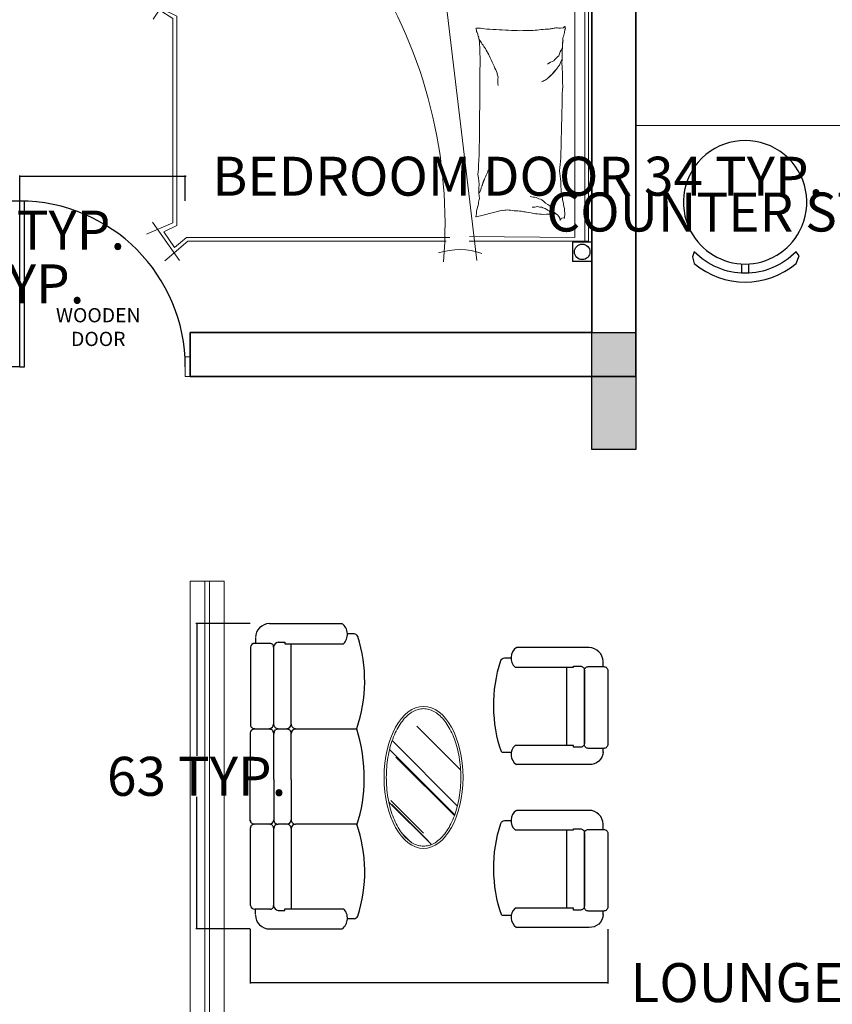
# Model space of a CAD drawing. Units: inches. Extents: x -48 to 50072, y 0 to 21068.
# Tile 68 of 75: x 925 to 1092, y 803 to 1005. Entities that reach past the tile are written whole.
import ezdxf

# ---------------------------------------------------------------- set-up
doc = ezdxf.new("R2010")
doc.units = ezdxf.units.IN
doc.header["$MEASUREMENT"] = 0
for name, color, linetype in [('2D', 7, 'Continuous'), ('BLOCKS', 7, 'Continuous'), ('家具1', 1, 'Continuous'), ('家具１', 1, 'Continuous')]:
    doc.layers.add(name, color=color, linetype=linetype)
for name, color, linetype, lineweight in [('A-ANNO-DIMS', 2, 'Continuous', 18), ('A-COLS', 1, 'Continuous', 35), ('A-DOOR', 4, 'Continuous', 18), ('A-FLOR-CASE', 9, 'Continuous', 18), ('A-FLOR-SCRN', 32, 'Continuous', 18), ('A-WALL', 7, 'Continuous', 35), ('FURNITURE', 44, 'Continuous', 18)]:
    doc.layers.add(name, color=color, linetype=linetype, lineweight=lineweight)
doc.styles.get("Standard").update_dxf_attribs({"font": 'arial.ttf'})
doc.dimstyles.get("Standard").update_dxf_attribs({"dimtxt": 8, "dimasz": 0.18, "dimexe": 0.18, "dimexo": 0.0625, "dimgap": 0.09, "dimtad": 0, "dimtih": 1, "dimtoh": 1, "dimdec": 1, "dimzin": 0, "dimdsep": 46, "dimlunit": 4, "dimtxsty": 'Standard', "dimblk": 'ARCHTICK', "dimcen": 0.09, "dimadec": 0, "dimazin": 0, "dimtfac": 1, "dimtdec": 1, "dimtofl": 0, "dimtmove": 0, "dimatfit": 3, "dimldrblk": 'ARCHTICK', "dimfxl": 1, "dimtolj": 1, "dimtzin": 0, "dimarcsym": 0})

# ---------------------------------------------------------------- blocks, each defined once
blk = doc.blocks.new('BKUHJKKUG')
at = {"layer": 'Defpoints'}
for p, q in [((179.52, 862.77), (179.52, 896.77)), ((180.52, 862.77), (180.52, 896.76)), ((179.52, 862.77), (180.52, 862.77))]:
    blk.add_line(p, q, dxfattribs=at)
blk.add_arc((179.52, 862.77), 34, 0, 90, dxfattribs=at)
at = {"insert": (190.84, 874.8), "char_height": 2.9183, "attachment_point": 1}
blk.add_mtext_dynamic_manual_height_columns('\\pxqc;WOODEN ^JDOOR', width=9.6242, gutter_width=14.59, heights=[0], dxfattribs=at)
blk = doc.blocks.new('bnniku')
at = {"layer": 'Defpoints'}
h = blk.add_hatch(color=256, dxfattribs=at)
h.dxf.hatch_style = 1
h.paths.add_polyline_path([(767.55, 1114.04), (758.55, 1114.04), (758.55, 1090.04), (767.55, 1090.04)])
for p, q in [((758.55, 1114.04), (767.55, 1114.04)), ((758.55, 1090.04), (758.55, 1114.04)), ((767.55, 1114.04), (767.55, 1090.04)), ((767.55, 1090.04), (758.55, 1090.04))]:
    blk.add_line(p, q, dxfattribs=at)
blk = doc.blocks.new('A$C78527CD7')
at = {"layer": 'BLOCKS'}
for p, q in [((119, 897.8), (162.3, 897.8)), ((162.3, 776.5), (162.3, 904.6)), ((194.3, 940.6), (831.7, 940.6)), ((862.2, 785.1), (862.2, 908.9)), ((886.4, 941), (1230.1, 941)), ((1611.9, 941), (1230.1, 941)), ((1644, 785.1), (1644, 908.9)), ((2316.1, 940.8), (1678.7, 940.8)), ((2348.2, 776.7), (2348.2, 904.9)), ((2391.5, 898), (2348.2, 898)), ((0, 783.4), (0, 188.4)), ((189.7, 748.7), (825.8, 748.7)), ((1230.1, 748.7), (886.4, 748.7)), ((1230.1, 748.7), (1611.9, 748.7)), ((2320.7, 749), (1684.6, 749)), ((2510.5, 783.6), (2510.5, 188.7)), ((152.6, 712.4), (152.6, 656.4)), ((152.6, 656.4), (166.9, 656.4)), ((166.9, 656.4), (166.9, 174.7)), ((862.2, 641.1), (862.2, 712.3)), ((1644, 641.1), (1644, 712.3)), ((2357.9, 656.7), (2343.6, 656.7)), ((2343.6, 656.7), (2343.6, 174.9)), ((2357.9, 712.6), (2357.9, 656.7)), ((825.8, 604.7), (166.9, 604.7)), ((862.2, 64.7), (862.2, 568.3)), ((1230.1, 604.7), (890.8, 604.7)), ((1230.1, 604.7), (1607.6, 604.7)), ((1644, 64.7), (1644, 568.3)), ((1684.6, 605), (2343.6, 605)), ((84.4, 88), (84.4, 142.7)), ((2426, 88.2), (2426, 142.9))]:
    blk.add_line(p, q, dxfattribs=at)
for centre, radius, start, end in [((114.4, 783.4), 114.4, 90, 180), ((197.9, 905.2), 35.6, 95.74502, 180.88345), ((829.5, 907.9), 32.8, 354.28815, 86.11137), ((894.3, 908.9), 32, 90, 180), ((1611.9, 908.9), 32, 0, 90), ((1680.9, 908.1), 32.8, 93.88863, 185.71185), ((2312.6, 905.4), 35.6, 359.11655, 84.25498), ((2396, 783.6), 114.4, 0, 90), ((203.8, 697.4), 53.9, 104.31345, 163.90285), ((190.2, 777.3), 27.9, 181.70275, 278.5003), ((825.8, 785.1), 36.4, 270, 360), ((825.8, 712.3), 36.4, 360, 90), ((898.6, 785.1), 36.4, 180, 270), ((898.6, 785.1), 36.4, 180, 270), ((898.6, 712.3), 36.4, 90, 180), ((1607.6, 785.1), 36.4, 270, 0), ((1607.6, 785.1), 36.4, 270, 0), ((1607.6, 712.3), 36.4, 0, 90), ((1684.6, 785.4), 36.4, 180, 270), ((1684.6, 712.6), 36.4, 90, 180), ((2320.3, 777.6), 27.9, 261.4997, 358.29725), ((2306.6, 697.7), 53.9, 16.09715, 75.68655), ((825.8, 641.1), 36.4, 270, 360), ((825.8, 568.3), 36.4, 360, 90), ((898.6, 641.1), 36.4, 180, 270), ((898.6, 568.3), 36.4, 90, 180), ((1607.6, 641.1), 36.4, 270, 0), ((1607.6, 568.3), 36.4, 0, 90), ((1684.6, 641.4), 36.4, 180, 270), ((1684.6, 568.6), 36.4, 90, 180), ((88.2, 253.3), 111.2, 217.55024, 315.04859), ((2422.3, 253.5), 111.2, 224.95141, 322.44976), ((116.5, 88), 32, 180, 252.1304), ((2394, 88.2), 32, 287.8696, 0), ((473.6, 1195.6), 1195.8, 252.1304, 288.99111), ((1223.2, 1157.8), 1153.7, 251.35305, 270.34112), ((1237.9, 1396), 1391.8, 269.68008, 286.96386), ((2036.9, 1195.8), 1195.8, 251.00889, 287.8696)]:
    blk.add_arc(centre, radius, start, end, dxfattribs=at)
blk = doc.blocks.new('A$C306A54D5')
for p, q in [((1089.2, 1060.9), (1351, 1322.4)), ((1177.4, 914.8), (1567.7, 1305)), ((1232.4, 898.4), (1621.3, 1287.3)), ((1275.1, 935.7), (1625.2, 1285.9)), ((1543.9, 893.1), (1798.6, 1147.8)), ((1558.5, 910.9), (1776.7, 1129.1)), ((1534.5, 904.5), (1730.5, 1100.5)), ((1728, 969.6), (1781.9, 1023.6))]:
    blk.add_line(p, q)
blk.add_ellipse((1396.6, 1101), major_axis=(-424.8, 0), ratio=0.556174)
blk.add_open_spline([(985.2, 1101), (985.2, 1090.7), (986.6, 1080.3), (992, 1059.7), (996.1, 1049.5), (1007.1, 1029.2), (1014, 1019.1), (1030.5, 999.6), (1040.1, 990.1), (1061.9, 971.8), (1074, 963), (1100.6, 946.5), (1115.1, 938.7), (1146, 924.4), (1162.4, 917.9), (1196.9, 906.2), (1214.9, 901), (1252.2, 892.2), (1271.5, 888.6), (1310.8, 882.8), (1330.8, 880.8), (1371.2, 878.3), (1391.6, 877.9), (1432.2, 878.7), (1452.5, 880), (1492.4, 884.1), (1512.1, 886.9), (1550.5, 894.2), (1569.2, 898.7), (1605.2, 908.9), (1622.5, 914.8), (1655.3, 927.9), (1670.8, 935), (1699.6, 950.5), (1712.9, 958.8), (1737.2, 976.3), (1748.1, 985.4), (1767.2, 1004.4), (1775.5, 1014.2), (1789.2, 1034.2), (1794.7, 1044.4), (1802.9, 1064.9), (1805.6, 1075.2), (1808.4, 1095.9), (1808.4, 1106.2), (1805.6, 1126.9), (1802.9, 1137.2), (1794.7, 1157.7), (1789.2, 1167.8), (1775.4, 1187.8), (1767.2, 1197.6), (1748, 1216.6), (1737.1, 1225.8), (1712.8, 1243.3), (1699.5, 1251.6), (1670.6, 1267), (1655.2, 1274.2), (1622.4, 1287.2), (1605.1, 1293.1), (1569.1, 1303.4), (1550.4, 1307.8), (1512, 1315.1), (1492.3, 1317.9), (1452.3, 1322), (1432.1, 1323.3), (1391.4, 1324.1), (1371.1, 1323.7), (1330.7, 1321.2), (1310.6, 1319.1), (1271.3, 1313.4), (1252.1, 1309.8), (1214.8, 1300.9), (1196.8, 1295.8), (1162.3, 1284.1), (1145.9, 1277.5), (1115, 1263.2), (1100.5, 1255.5), (1073.9, 1238.9), (1061.8, 1230.2), (1040, 1211.9), (1030.4, 1202.3), (1013.9, 1182.8), (1007.1, 1172.8), (996.1, 1152.5), (992, 1142.2), (986.6, 1121.6), (985.2, 1111.3), (985.2, 1101)], degree=3, knots=[0, 0, 0, 0, 0.146129, 0.146129, 0.292258, 0.292258, 0.438387, 0.438387, 0.584516, 0.584516, 0.730645, 0.730645, 0.876774, 0.876774, 1.022902, 1.022902, 1.169031, 1.169031, 1.31516, 1.31516, 1.461289, 1.461289, 1.607418, 1.607418, 1.753547, 1.753547, 1.899676, 1.899676, 2.045805, 2.045805, 2.191934, 2.191934, 2.338063, 2.338063, 2.484192, 2.484192, 2.630321, 2.630321, 2.77645, 2.77645, 2.922579, 2.922579, 3.068707, 3.068707, 3.214836, 3.214836, 3.360965, 3.360965, 3.507094, 3.507094, 3.653223, 3.653223, 3.799352, 3.799352, 3.945481, 3.945481, 4.09161, 4.09161, 4.237739, 4.237739, 4.383868, 4.383868, 4.529997, 4.529997, 4.676126, 4.676126, 4.822255, 4.822255, 4.968383, 4.968383, 5.114512, 5.114512, 5.260641, 5.260641, 5.40677, 5.40677, 5.552899, 5.552899, 5.699028, 5.699028, 5.845157, 5.845157, 5.991286, 5.991286, 6.137415, 6.137415, 6.283185, 6.283185, 6.283185, 6.283185])
at = {"layer": 'BLOCKS'}
for p, q in [((1246.7, 2175.3), (1222.7, 2175.3)), ((2220.4, 2175.3), (2196.4, 2175.3)), ((1206, 1958.7), (737.3, 1958.7)), ((2179.7, 1958.7), (1710.9, 1958.7)), ((1248.5, 1625.2), (1248.5, 1572)), ((2222.2, 1625.2), (2222.2, 1572))]:
    blk.add_line(p, q, dxfattribs=at)
for points in [[(757.3, 2063.6, -0.414214), (733.9, 2086.9), (733.9, 2180.2, -0.414214), (757.3, 2203.6), (1199.4, 2203.6, -0.414214), (1222.7, 2180.2), (1222.7, 2086.9, -0.414214), (1199.4, 2063.6)], [(1730.9, 2063.6, -0.414214), (1707.6, 2086.9), (1707.6, 2180.2, -0.414214), (1730.9, 2203.6), (2173, 2203.6, -0.414214), (2196.4, 2180.2), (2196.4, 2086.9, -0.414214), (2173, 2063.6)]]:
    blk.add_lwpolyline(points, format="xyb", close=True, dxfattribs=at)
for points in [[(733.9, 2175.3), (703.6, 2175.3, 0.414214), (620.2, 2091.9), (620.2, 1658.6)], [(1244.2, 2175.3, -0.433237), (1320, 2091.9), (1320, 1658.6)], [(1707.6, 2175.3), (1677.2, 2175.3, 0.414214), (1593.9, 2091.9), (1593.9, 1658.6)], [(2217.9, 2175.3, -0.433237), (2293.7, 2091.9), (2293.7, 1658.6)], [(620.2, 1656.5, 0.470418), (737.3, 1648.6), (737.3, 1999.5), (731.1, 1999.5), (731.1, 2040.2, -0.414214), (754.5, 2063.6), (1193.1, 2063.6, -0.414214), (1216.4, 2040.2), (1216.4, 1999.5), (1206, 1999.5), (1206, 1648.6, 0.482727), (1320, 1656.5)], [(1593.9, 1656.5, 0.470418), (1710.9, 1648.6), (1710.9, 1999.5), (1704.8, 1999.5), (1704.8, 2040.2, -0.414214), (1728.1, 2063.6), (2166.7, 2063.6, -0.414214), (2190.1, 2040.2), (2190.1, 1999.5), (2179.7, 1999.5), (2179.7, 1648.6, 0.482727), (2293.7, 1656.5)], [(1248.5, 1568.7, -0.162236), (697.9, 1563.3, -0.325549), (681.7, 1585.5), (681.7, 1625.3)], [(2222.2, 1568.7, -0.162236), (1671.6, 1563.3, -0.325549), (1655.4, 1585.5), (1655.4, 1625.3)]]:
    blk.add_lwpolyline(points, format="xyb", dxfattribs=at)
at = {"xscale": 0.7278252318920257, "yscale": 0.7278252318920257, "zscale": 0.7278252318920257, "rotation": 180}
blk.add_blockref('A$C78527CD7', (2303.6, 748.9), dxfattribs=at)
blk = doc.blocks.new('A$C7A8469D8')
for p, q in [((105.4, 2275.5), (1345.4, 2275.5)), ((105.4, 1660.8), (105.4, 2275.5)), ((1345.4, 2255.5), (105.4, 2255.5)), ((1345.4, 2275.5), (1345.4, 1540.4)), ((3363.9, 2275.5), (2123.9, 2275.5)), ((2123.9, 2275.5), (2123.9, 1540.4)), ((2123.9, 2255.5), (3363.9, 2255.5)), ((3363.9, 1660.8), (3363.9, 2275.5)), ((1325.4, 2205.5), (125.4, 2205.5)), ((129.2, 1662.5), (125.4, 2205.5)), ((1325.4, 1539.2), (1325.4, 2205.5)), ((2143.9, 2205.5), (3343.9, 2205.5)), ((2143.9, 1539.2), (2143.9, 2205.5)), ((3340.1, 1662.5), (3343.9, 2205.5)), ((963.7, 2086.6), (963.7, 2086.6)), ((963.7, 2086.6), (963.7, 2086.6)), ((997.2, 2115.8), (997.2, 2115.8)), ((2472.1, 2115.8), (2472.1, 2115.8)), ((2505.6, 2086.6), (2505.6, 2086.6)), ((2505.6, 2086.6), (2505.6, 2086.6)), ((940.8, 2061.8), (940.8, 2061.8)), ((2528.5, 2061.8), (2528.5, 2061.8)), ((284, 2013), (284, 2013)), ((284, 2013), (284, 2013)), ((3185.3, 2013), (3185.3, 2013)), ((3185.3, 2013), (3185.3, 2013)), ((239.9, 1733), (264.7, 1832.1)), ((3229.5, 1733), (3204.7, 1832.1)), ((230.9, 1697), (239.9, 1733)), ((1064.8, 1762.3), (1064.8, 1762.3)), ((1096.9, 1744.2), (1096.9, 1744.2)), ((1096.9, 1744.2), (1096.9, 1744.2)), ((1096.9, 1744.2), (1096.9, 1744.2)), ((2372.4, 1744.2), (2372.4, 1744.2)), ((2372.4, 1744.2), (2372.4, 1744.2)), ((2372.4, 1744.2), (2372.4, 1744.2)), ((2404.5, 1762.3), (2404.5, 1762.3)), ((3238.5, 1697), (3229.5, 1733)), ((1476.1, 1524.8), (6.4, 1700.6)), ((230.9, 1697), (230.5, 1695.5)), ((1993.2, 1524.8), (3462.9, 1700.6)), ((3238.5, 1697), (3238.8, 1695.5)), ((105.4, 212.1), (105.4, 1542.9)), ((125.4, 204.7), (125.4, 1561.6)), ((3343.9, 204.7), (3343.9, 1561.6)), ((3363.9, 212.1), (3363.9, 1542.9)), ((1325.4, 204.7), (1325.4, 1280.1)), ((2143.9, 204.7), (2143.9, 1280.1)), ((1345.4, 1261.4), (1345.4, 212.1)), ((2123.9, 1261.4), (2123.9, 212.1)), ((4.4, 94.3), (105.4, 212.1)), ((125.4, 204.7), (73.3, 144)), ((1325.4, 204.7), (1377.6, 144)), ((1345.4, 212.1), (1446.2, 92.2)), ((2123.9, 212.1), (2023.1, 92.2)), ((2143.9, 204.7), (2091.7, 144)), ((3343.9, 204.7), (3396, 144)), ((3464.9, 94.3), (3363.9, 212.1)), ((203.9, 30), (6.6, 169.4)), ((154.5, 88.5), (186.9, 155.5)), ((186.9, 155.5), (1264, 155.5)), ((1452.6, 169.4), (1248.8, 34.3)), ((1296.4, 88.5), (1264, 155.5)), ((2016.7, 169.4), (2220.5, 34.3)), ((2172.9, 88.5), (2205.3, 155.5)), ((3282.4, 155.5), (2205.3, 155.5)), ((3265.4, 30), (3462.8, 169.4)), ((3314.8, 88.5), (3282.4, 155.5)), ((73.3, 144), (154.5, 88.5)), ((199.5, 135.5), (141.7, 0)), ((1251.4, 135.5), (199.5, 135.5)), ((1323.9, 21.4), (1251.4, 135.5)), ((1377.6, 144), (1296.4, 88.5)), ((2091.7, 144), (2172.9, 88.5)), ((2145.4, 21.4), (2217.9, 135.5)), ((2217.9, 135.5), (3269.8, 135.5)), ((3269.8, 135.5), (3327.6, 0)), ((3396, 144), (3314.8, 88.5))]:
    blk.add_line(p, q)
for centre, radius, start, end in [((227.2, 2136.4), 15.7, 101.2724, 206.5805), ((249.8, 2147.7), 41, 206.5805, 265.5998), ((245.3, 2045.5), 108.5, 90, 101.2724), ((245.3, 1960.6), 193.4, 81.5628, 90), ((220, 1790.1), 365.7, 74.256, 81.5628), ((398.1, 2421.9), 290.7, 254.256, 262.4531), ((467.5, 2945.8), 819.2, 262.4531, 270), ((467.5, 3385.4), 1258.8, 270, 276.0867), ((201.4, 24611.4), 22481.3, 271.01841, 271.70805), ((903.9, 1960.2), 182.9, 92.5386, 100.1899), ((911.2, 1795.5), 347.6, 85.1982, 92.5386), ((1028, 3186.1), 1047.8, 265.1982, 269.4243), ((1140.8, 1875.8), 280.8, 110.8603, 117.2396), ((1035.5, 3931.4), 1793.1, 269.4243, 271.9079), ((1130.4, 2026.4), 119, 105.9352, 126.0864), ((1062.4, 3123.6), 984.9, 271.9079, 275.2592), ((1130.4, 2026.4), 119, 85.7841, 105.9352), ((1146.7, 2207.3), 64.7, 275.2592, 300.6513), ((1197.4, 2121.8), 34.7, 85.6975, 120.6513), ((1197.7, 2126.3), 30.1, 68.2117, 85.6975), ((1219.6, 2138.1), 18.7, 158.0096, 201.421), ((1207, 2143.2), 5.13, 78.1069, 158.0096), ((1165.5, 2116.9), 39.3, 351.8665, 21.421), ((1208.6, 2150.9), 2.78, 258.1069, 19.564), ((1207.4, 2150.5), 4.1, 19.564, 68.2117), ((2256.5, 2155.7), 4.1, 291.7883, 340.436), ((2258.6, 2149.1), 2.78, 340.436, 101.8931), ((2258.1, 2184.3), 30.1, 274.3025, 291.7883), ((2266, 2150.1), 5.13, 201.9904, 281.8931), ((2228.2, 2125.7), 39.3, 338.579, 8.1335), ((2284.5, 2138.3), 18.7, 158.579, 201.9904), ((2287, 2186.2), 34.7, 239.3487, 274.3025), ((2283.7, 2087.2), 64.7, 59.3487, 84.7408), ((2283.9, 1158.4), 984.9, 84.7408, 88.0921), ((2362.9, 2259.6), 119, 254.0648, 274.2159), ((2441.7, 2237), 119, 233.9136, 254.0648), ((2392.2, 346.2), 1793.1, 88.0921, 90.5757), ((2557.1, 2387.9), 280.8, 242.7604, 249.1397), ((2539.6, 1094.2), 1047.8, 90.5757, 94.8018), ((2544.4, 2489.3), 347.6, 267.4614, 274.8018), ((2605.9, 2322.8), 182.9, 259.8101, 267.4614), ((2198.2, -20337.6), 22481.3, 88.29195, 88.98159), ((2868.3, 874.9), 1258.8, 83.9133, 90), ((3109.4, 1314.5), 819.2, 90, 97.5469), ((3188.3, 1853.9), 290.7, 97.5469, 105.744), ((3096.4, 2503.8), 365.7, 278.4372, 285.744), ((3195.6, 2345.2), 193.4, 270, 278.4372), ((3259.4, 2088.4), 41, 94.4002, 153.4195), ((3245.2, 2260.3), 108.5, 258.7276, 270), ((3259.3, 2144.8), 15.7, 153.4195, 258.7276), ((833.2, 2043.1), 590.2, 173.7676, 180), ((180.9, 2000.6), 107.8, 41.4429, 53.7359), ((169.6, 1957.5), 167.9, 45.0976, 62.7964), ((1150.7, 1891.6), 270.2, 133.8115, 140.9651), ((1150.7, 1891.6), 270.2, 133.8115, 140.9651), ((1150.7, 1891.6), 270.2, 133.8115, 140.9651), ((1289, 1747.4), 470, 128.3886, 133.8115), ((1289, 1747.4), 470, 128.3886, 133.8115), ((1289, 1747.4), 470, 128.3886, 133.8115), ((1054.4, 2043.6), 92.1, 117.2396, 128.3886), ((1130.4, 2026.4), 119, 143.8234, 161.5603), ((1130.4, 2026.4), 119, 126.0864, 143.8234), ((1433.6, 2041.2), 238, 167.8905, 172.3191), ((912.2, 2153.1), 295.2, 347.8905, 351.8665), ((1976.2, 2049.4), 295.2, 8.1335, 12.1095), ((2504.3, 2123), 238, 187.6809, 192.1095), ((2505.1, 2192.8), 119, 216.1766, 233.9136), ((2548, 2134.3), 119, 198.4397, 216.1766), ((2514.3, 2197.7), 92.1, 231.6114, 242.7604), ((2797.5, 2455), 470, 226.1885, 231.6114), ((2180.3, 1747.4), 470, 46.1885, 51.6114), ((2180.3, 1747.4), 470, 46.1885, 51.6114), ((2715.6, 2256.8), 270.2, 219.0349, 226.1885), ((2318.6, 1891.6), 270.2, 39.0349, 46.1885), ((2318.6, 1891.6), 270.2, 39.0349, 46.1885), ((3104.4, 2225.8), 167.9, 297.2036, 314.9024), ((3143.8, 2159), 107.8, 306.2641, 318.5571), ((3813.1, 2107.2), 590.2, 180, 186.2324), ((487.7, 2043.1), 244.8, 180, 189.6844), ((214.4, 2030.2), 63.1, 25.3551, 41.4429), ((107.6, 1979.6), 181.3, 21.8149, 25.3551), ((46.9, 1955.3), 246.7, 18.7799, 21.8149), ((216.6, 2013), 67.4, 0, 18.7799), ((169.6, 1957.5), 167.9, 27.3988, 45.0976), ((169.6, 1957.5), 167.9, 16.515, 27.3988), ((1146.2, 1938.6), 240.2, 151.6832, 156.9972), ((986.8, 2024.5), 59.2, 140.9651, 151.6832), ((2283.6, 1926.6), 1095.7, 172.3191, 176.6313), ((3365.4, 2137.4), 1095.7, 183.3687, 187.6809), ((2580.6, 2089.8), 59.2, 208.3168, 219.0349), ((2755.7, 2146.4), 240.2, 203.0028, 208.3168), ((2989.6, 2082.5), 167.9, 332.6012, 343.485), ((3032, 2153.7), 167.9, 314.9024, 332.6012), ((3121.5, 2034.7), 67.4, 341.2201, 360), ((2959.9, 2126.4), 246.7, 338.1851, 341.2201), ((3029.6, 2124.6), 181.3, 334.6449, 338.1851), ((3150.6, 2099), 63.1, 318.5571, 334.6449), ((3467.6, 2001.9), 244.8, 170.3156, 180), ((1289.8, 2180), 1058.4, 189.6844, 192.1984), ((174.2, 2013), 109.8, 345.3149, 360), ((169.6, 1957.5), 167.9, 5.6311, 16.515), ((2002.9, 1943.1), 814.5, 176.6313, 181.6331), ((3093.7, 1967.8), 814.5, 178.3669, 183.3687), ((2971.5, 2021.7), 167.9, 343.485, 354.3689), ((3079.1, 1985.2), 109.8, 0, 14.6851), ((4257.4, 1778.3), 1058.4, 167.8016, 170.3156), ((-116.7, 1875.9), 380.5, 8.0051, 12.1984), ((-522.7, 1818.8), 790.5, 2.6649, 8.0051), ((2419.5, 1965.7), 790.5, 351.9949, 357.3351), ((2837.2, 2009.3), 380.5, 347.8016, 351.9949), ((2826.3, 1966.6), 1638.3, 181.6331, 183.055), ((17529.8, 2751.3), 16362.7, 183.05496, 183.50486), ((18611, 879), 16362.7, 176.49514, 176.94504), ((3916.5, 1832.6), 1638.3, 176.945, 178.3669), ((185.8, 1851.8), 81.3, 345.9548, 2.6649), ((3123.5, 1835.8), 81.3, 357.3351, 14.0452), ((927.3, 1483.7), 326.5, 85.9172, 93.5552), ((945.6, 1740), 69.6, 69.3257, 85.9172), ((755.5, 1236.2), 608, 65.6735, 69.3257), ((297.9, 224.1), 1718.7, 63.5015, 65.6735), ((1696.5, 3328.4), 1718.7, 294.3265, 296.4985), ((2248.7, 2359), 608, 290.6743, 294.3265), ((2494.2, 1874.4), 69.6, 274.0828, 290.6743), ((2539, 2135.2), 326.5, 266.4448, 274.0828), ((-288.1, 1611.6), 350.3, 341.9888, 19.1136), ((93, 2561.3), 886.4, 287.1982, 289.428), ((93, 2561.3), 886.4, 289.4267, 291.8864), ((93, 2561.3), 886.4, 289.428, 291.6577), ((93, 2561.3), 886.4, 289.4283, 291.559), ((93, 2561.3), 886.4, 289.4267, 289.4283), ((93, 2561.3), 886.4, 291.43, 291.7259), ((93, 2561.3), 886.4, 291.43, 291.71), ((93, 2561.3), 886.4, 291.443, 291.8345), ((93, 2561.3), 886.4, 291.443, 291.484), ((93, 2561.3), 886.4, 291.484, 291.7259), ((93, 2561.3), 886.4, 291.559, 291.8345), ((93, 2561.3), 886.4, 291.6577, 293.4844), ((93, 2561.3), 886.4, 291.71, 291.8864), ((93, 2561.3), 886.4, 293.4844, 295.3111), ((897.4, 1426.5), 375.2, 57.865, 63.5015), ((897.4, 1426.5), 375.2, 57.865, 63.5015), ((897.4, 1426.5), 375.2, 57.865, 63.5015), ((631.9, 1003.8), 874.3, 54.1737, 57.865), ((1582.4, 1774.6), 385.4, 183.5049, 189.9984), ((2651.1, 1684.1), 385.4, 170.0016, 176.4951), ((1860.6, 2453.1), 874.3, 302.135, 305.8263), ((2205, 2080), 375.2, 296.4985, 302.135), ((2571.9, 1426.5), 375.2, 116.4985, 122.135), ((2571.9, 1426.5), 375.2, 116.4985, 122.135), ((2644.1, 947), 886.4, 64.6889, 66.5156), ((2695.9, 924.5), 886.4, 66.5156, 68.3423), ((3376.3, 2561.3), 886.4, 248.1136, 250.5733), ((3376.3, 2561.3), 886.4, 248.1136, 248.29), ((3376.3, 2561.3), 886.4, 248.1655, 248.557), ((3376.3, 2561.3), 886.4, 248.1655, 248.441), ((3376.3, 2561.3), 886.4, 248.2741, 248.57), ((3376.3, 2561.3), 886.4, 248.2741, 248.516), ((3376.3, 2561.3), 886.4, 248.29, 248.57), ((2754.3, 901.6), 886.4, 68.3423, 70.572), ((3376.3, 2561.3), 886.4, 248.441, 250.5717), ((3376.3, 2561.3), 886.4, 248.516, 248.557), ((3376.3, 2561.3), 886.4, 250.5717, 250.5733), ((2819.4, 878.6), 886.4, 70.572, 72.8018), ((3757.4, 1611.6), 350.3, 160.8864, 198.0112), ((208.9, 2019.7), 324.9, 273.8155, 274.0829), ((231.9, 1696.7), 1.1, 165.9546, 274.0829), ((231.9, 1696.7), 1.1, 165.9551, 274.0829), ((208.9, 2019.7), 324.9, 274.0829, 279.4841), ((217, 1971), 275.6, 279.4841, 287.3864), ((342.3, 1570.9), 143.7, 96.4341, 107.3864), ((345.8, 1539.7), 175.1, 78.4414, 96.4341), ((436.2, 1981.7), 276.1, 258.4414, 272.7491), ((368.6, 3389.7), 1685.7, 272.7491, 274.6176), ((621.8, 254.5), 1459.7, 92.6096, 94.6176), ((1098, -33470.9), 35187.8, 90.32849, 90.88356), ((1012.4, -5144.9), 6862.2, 89.71346, 90.97038), ((1039.8, 320.4), 1396.8, 86.426, 89.7135), ((1115.9, 1539.8), 175.1, 77.131, 86.426), ((1142.8, 1657.5), 54.3, 62.7159, 77.131), ((1209.9, 1787.6), 92.1, 242.7159, 253.7788), ((1213.5, 1800), 105, 253.7788, 262.8796), ((1200.7, 1697.4), 1.59, 262.8796, 343.3022), ((1180, 1703.6), 23.2, 343.3022, 9.9984), ((2244.2, 1701), 23.2, 350.0016, 16.6978), ((2267.3, 1695.4), 1.59, 16.6978, 97.1204), ((2298.1, 1595), 105, 97.1204, 106.2212), ((2327.3, 1617.4), 92.1, 106.2212, 117.2841), ((2289.5, 1758.8), 54.3, 282.869, 297.2841), ((2303.5, 1885.2), 175.1, 273.574, 282.869), ((2335.5, 3111.3), 1396.8, 270.2865, 273.574), ((2538.8, 8578.4), 6862.2, 269.02962, 270.28654), ((3115.7, 36899.9), 35187.8, 269.11644, 269.67151), ((3031.5, 3167.7), 1459.7, 265.3824, 267.3904), ((2884.2, 25.7), 1685.7, 85.3824, 87.2509), ((3075.2, 1435.5), 276.1, 87.2509, 101.5586), ((3108.1, 1885.2), 175.1, 263.5659, 281.5586), ((3186.1, 1850.8), 143.7, 252.6136, 263.5659), ((3124.6, 1436.2), 275.6, 72.6136, 80.5159), ((3183.8, 1375.1), 324.9, 80.5159, 85.9171), ((3237.4, 1696.7), 1.1, 265.9171, 14.0454), ((3238.4, 1695.9), 1.1, 85.9171, 194.0449), ((3260.5, 2019.7), 324.9, 265.9171, 266.1845), ((2296.9, 1493), 913.1, 173.1442, 204.7336), ((1172.5, 1493), 913.1, 335.2664, 6.8558), ((191.6, -937), 2473.5, 57.4247, 94.4416), ((3277.8, -937), 2473.5, 85.5584, 122.5753)]:
    blk.add_arc(centre, radius, start, end)
at = {"layer": '家具1'}
for p, q in [((100.7, 2292.6), (0.7, 2292.6)), ((0.7, 2292.6), (0.7, 2192.6)), ((100.7, 2292.6), (100.7, 2192.6)), ((1348.1, 2292.6), (1448.1, 2292.6)), ((1348.1, 2292.6), (1348.1, 2192.6)), ((2031.9, 2292.6), (1440.5, 2292.6)), ((1448.1, 2303.2), (1448.1, 1885)), ((1448.1, 2292.6), (1448.1, 2192.6)), ((1613.7, 2082.3), (1613.7, 2329.8)), ((1836.1, 2082.3), (1836.1, 2329.8)), ((2018.1, 2303.2), (2018.1, 1885)), ((2121.2, 2292.6), (2021.2, 2292.6)), ((2021.2, 2292.6), (2021.2, 2192.6)), ((2121.2, 2292.6), (2121.2, 2192.6)), ((3368.6, 2292.6), (3468.6, 2292.6)), ((3368.6, 2292.6), (3368.6, 2192.6)), ((100.7, 2192.6), (0.7, 2192.6)), ((1348.1, 2192.6), (1448.1, 2192.6)), ((1518.4, 2196.5), (1709, 2196.5)), ((1757, 2205.5), (1695.7, 2205.5)), ((1757, 2185.5), (1695.7, 2185.5)), ((1740.8, 2196.5), (1931.4, 2196.5)), ((2121.2, 2192.6), (2021.2, 2192.6)), ((3368.6, 2192.6), (3468.6, 2192.6)), ((2028.8, 1892.6), (1440.5, 1892.6)), ((1448.1, 1792.9), (1448.1, 260.3)), ((2018.1, 1787.6), (2018.1, 260.3)), ((2028.8, 1767.9), (1440.5, 1767.9)), ((2028.8, 267.9), (1440.5, 267.9))]:
    blk.add_line(p, q, dxfattribs=at)
for centre, radius in [((50.7, 2242.6), 40), ((1398.1, 2242.6), 40), ((2071.2, 2242.6), 40), ((3418.6, 2242.6), 40), ((1616.3, 2195.5), 80), ((1836.3, 2195.5), 80)]:
    blk.add_circle(centre, radius, dxfattribs=at)
at = {"layer": '家具１'}
blk.add_line((3468.6, 2292.6), (3468.6, 2192.6), dxfattribs=at)
blk = doc.blocks.new('A$C4C1A535A')
at = {"layer": '2D'}
for p, q in [((298.3, 92.9), (298.3, 45.3)), ((334.4, 92.9), (334.4, 45.3))]:
    blk.add_line(p, q, dxfattribs=at)
for points in [[(37, 260, 0.600226), (595.8, 260, 1.666039)], [(577.7, 155.5, -0.423227), (55, 155.5), (47.1, 129.3), (55, 94.4, 0.361278), (577.7, 94.4), (593.6, 134.5)]]:
    blk.add_lwpolyline(points, format="xyb", close=True, dxfattribs=at)
blk = doc.blocks.new('SCREEN-JALI-90')
for p, q in [((7, 90), (0, 90)), ((0, 90), (0, 0)), ((3, 90), (3, 0)), ((4, 90), (4, 0)), ((7, 0), (7, 90)), ((7, 0), (0, 0))]:
    blk.add_line(p, q)
blk = doc.blocks.new('_ArchTick')
at = {"color": 0, "linetype": 'ByBlock', "const_width": 0.15}
blk.add_lwpolyline([(-0.5, -0.5), (0.5, 0.5)], dxfattribs=at)
blk = doc.blocks.new('*D66')
at = {"layer": 'A-ANNO-DIMS', "color": 0, "lineweight": -2, "transparency": 16777216}
for p, q in [((924.76, 967.53), (924.76, 972.74)), ((924.76, 972.56), (958.76, 972.56)), ((958.76, 967.53), (958.76, 972.74)), ((958.76, 972.56), (958.94, 972.56))]:
    blk.add_line(p, q, dxfattribs=at)
at = {"layer": 'Defpoints', "color": 0, "transparency": 16777216}
for p in [(958.76, 972.56), (924.76, 967.46), (958.76, 967.46)]:
    blk.add_point(p, dxfattribs=at)
at = {"layer": 'A-ANNO-DIMS', "color": 0, "lineweight": -2, "transparency": 16777216, "xscale": 0.18, "yscale": 0.18, "zscale": 0.18, "rotation": 180}
blk.add_blockref('_ArchTick', (924.76, 972.56), dxfattribs=at)
at = {"layer": 'A-ANNO-DIMS', "color": 0, "lineweight": -2, "transparency": 16777216, "xscale": 0.18, "yscale": 0.18, "zscale": 0.18}
blk.add_blockref('_ArchTick', (958.76, 972.56), dxfattribs=at)
at = {"layer": 'A-ANNO-DIMS', "color": 0, "transparency": 16777216, "insert": (1027.07, 972.56), "char_height": 8, "attachment_point": 5}
blk.add_mtext('\\A1;BEDROOM DOOR 34 TYP.', dxfattribs=at)
blk = doc.blocks.new('*D67')
at = {"layer": 'A-ANNO-DIMS', "color": 0, "lineweight": -2, "transparency": 16777216}
for p, q in [((924.7, 967.46), (919.48, 967.46)), ((919.66, 967.46), (919.66, 954.64)), ((919.66, 933.46), (919.66, 946.29)), ((924.7, 933.46), (919.48, 933.46))]:
    blk.add_line(p, q, dxfattribs=at)
at = {"layer": 'Defpoints', "color": 0, "transparency": 16777216}
for p in [(919.66, 967.46), (924.76, 967.46), (924.76, 933.46)]:
    blk.add_point(p, dxfattribs=at)
at = {"layer": 'A-ANNO-DIMS', "color": 0, "lineweight": -2, "transparency": 16777216, "xscale": 0.18, "yscale": 0.18, "zscale": 0.18}
for p, rotation in [((919.66, 967.46), 90), ((919.66, 933.46), 270)]:
    blk.add_blockref('_ArchTick', p, dxfattribs=dict(at, rotation=rotation))
at = {"layer": 'A-ANNO-DIMS', "color": 0, "transparency": 16777216, "insert": (919.66, 950.46), "char_height": 8, "attachment_point": 5}
blk.add_mtext('\\A1;34 TYP.', dxfattribs=at)
blk = doc.blocks.new('*D76')
at = {"layer": 'A-ANNO-DIMS', "color": 0, "lineweight": -2, "transparency": 16777216}
for p, q in [((972.12, 817.98), (972.12, 806.85)), ((1045.51, 817.98), (1045.51, 806.85)), ((972.12, 807.03), (1045.51, 807.03)), ((1045.51, 807.03), (1045.69, 807.03))]:
    blk.add_line(p, q, dxfattribs=at)
at = {"layer": 'Defpoints', "color": 0, "transparency": 16777216}
for p in [(972.12, 818.04), (1045.51, 818.04), (1045.51, 807.03)]:
    blk.add_point(p, dxfattribs=at)
at = {"layer": 'A-ANNO-DIMS', "color": 0, "lineweight": -2, "transparency": 16777216, "xscale": 0.18, "yscale": 0.18, "zscale": 0.18, "rotation": 180}
blk.add_blockref('_ArchTick', (972.12, 807.03), dxfattribs=at)
at = {"layer": 'A-ANNO-DIMS', "color": 0, "lineweight": -2, "transparency": 16777216, "xscale": 0.18, "yscale": 0.18, "zscale": 0.18}
blk.add_blockref('_ArchTick', (1045.51, 807.03), dxfattribs=at)
at = {"layer": 'A-ANNO-DIMS', "color": 0, "transparency": 16777216, "insert": (1102.65, 807.03), "char_height": 8, "attachment_point": 5}
blk.add_mtext('\\A1;LOUNGE SET 73 TYP.', dxfattribs=at)
blk = doc.blocks.new('*D77')
at = {"layer": 'A-ANNO-DIMS', "color": 0, "lineweight": -2, "transparency": 16777216}
for p, q in [((972.06, 880.72), (960.93, 880.72)), ((961.11, 880.72), (961.11, 853.56)), ((961.11, 818.04), (961.11, 845.2)), ((972.06, 818.04), (960.93, 818.04))]:
    blk.add_line(p, q, dxfattribs=at)
at = {"layer": 'Defpoints', "color": 0, "transparency": 16777216}
for p in [(972.12, 880.72), (961.11, 818.04), (972.12, 818.04)]:
    blk.add_point(p, dxfattribs=at)
at = {"layer": 'A-ANNO-DIMS', "color": 0, "lineweight": -2, "transparency": 16777216, "xscale": 0.18, "yscale": 0.18, "zscale": 0.18}
for p, rotation in [((961.11, 880.72), 90), ((961.11, 818.04), 270)]:
    blk.add_blockref('_ArchTick', p, dxfattribs=dict(at, rotation=rotation))
at = {"layer": 'A-ANNO-DIMS', "color": 0, "transparency": 16777216, "insert": (961.11, 849.38), "char_height": 8, "attachment_point": 5}
blk.add_mtext('\\A1;63 TYP.', dxfattribs=at)
blk = doc.blocks.new('*D82')
at = {"layer": 'A-ANNO-DIMS', "color": 0, "lineweight": -2, "transparency": 16777216}
for p, q in [((877.31, 973.04), (880.89, 973.04)), ((880.71, 973.04), (880.71, 965.98)), ((880.71, 949.97), (880.71, 957.04)), ((877.31, 949.97), (880.89, 949.97))]:
    blk.add_line(p, q, dxfattribs=at)
at = {"layer": 'Defpoints', "color": 0, "transparency": 16777216}
for p in [(877.25, 973.04), (880.71, 973.04), (877.25, 949.97)]:
    blk.add_point(p, dxfattribs=at)
at = {"layer": 'A-ANNO-DIMS', "color": 0, "lineweight": -2, "transparency": 16777216, "xscale": 0.18, "yscale": 0.18, "zscale": 0.18}
for p, rotation in [((880.71, 973.04), 90), ((880.71, 949.97), 270)]:
    blk.add_blockref('_ArchTick', p, dxfattribs=dict(at, rotation=rotation))
at = {"layer": 'A-ANNO-DIMS', "color": 0, "transparency": 16777216, "insert": (880.71, 961.51), "char_height": 8, "attachment_point": 5}
blk.add_mtext('\\A1;DESK EQUIPMENT 23 TYP.', dxfattribs=at)
blk = doc.blocks.new('*D92')
at = {"layer": 'A-ANNO-DIMS', "color": 0, "lineweight": -2, "transparency": 16777216}
for p, q in [((1051.25, 1019.39), (1051.25, 1015.11)), ((1078.96, 1019.39), (1078.96, 1015.11)), ((1051.25, 1015.29), (1051.07, 1015.29)), ((1078.96, 1015.29), (1051.25, 1015.29))]:
    blk.add_line(p, q, dxfattribs=at)
at = {"layer": 'Defpoints', "color": 0, "transparency": 16777216}
for p in [(1051.25, 1019.45), (1078.96, 1019.45), (1051.25, 1015.29)]:
    blk.add_point(p, dxfattribs=at)
at = {"layer": 'A-ANNO-DIMS', "color": 0, "lineweight": -2, "transparency": 16777216, "xscale": 0.18, "yscale": 0.18, "zscale": 0.18, "rotation": 180}
blk.add_blockref('_ArchTick', (1051.25, 1015.29), dxfattribs=at)
at = {"layer": 'A-ANNO-DIMS', "color": 0, "lineweight": -2, "transparency": 16777216, "xscale": 0.18, "yscale": 0.18, "zscale": 0.18}
blk.add_blockref('_ArchTick', (1078.96, 1015.29), dxfattribs=at)
at = {"layer": 'A-ANNO-DIMS', "color": 0, "transparency": 16777216, "insert": (985.76, 1015.29), "char_height": 8, "attachment_point": 5}
blk.add_mtext('\\A1;REFRIGERATOR 28 TYP.', dxfattribs=at)
blk = doc.blocks.new('*D94')
at = {"layer": 'A-ANNO-DIMS', "color": 0, "lineweight": -2, "transparency": 16777216}
for p, q in [((1101.33, 980.84), (1096.52, 980.84)), ((1096.7, 980.84), (1096.7, 969.45)), ((1096.7, 949.58), (1096.7, 960.98)), ((1101.33, 949.58), (1096.52, 949.58))]:
    blk.add_line(p, q, dxfattribs=at)
at = {"layer": 'Defpoints', "color": 0, "transparency": 16777216}
for p in [(1096.7, 980.84), (1101.39, 980.84), (1101.39, 949.58)]:
    blk.add_point(p, dxfattribs=at)
at = {"layer": 'A-ANNO-DIMS', "color": 0, "lineweight": -2, "transparency": 16777216, "xscale": 0.18, "yscale": 0.18, "zscale": 0.18}
for p, rotation in [((1096.7, 980.84), 90), ((1096.7, 949.58), 270)]:
    blk.add_blockref('_ArchTick', p, dxfattribs=dict(at, rotation=rotation))
at = {"layer": 'A-ANNO-DIMS', "color": 0, "transparency": 16777216, "insert": (1096.7, 965.21), "char_height": 8, "attachment_point": 5}
blk.add_mtext('\\A1;COUNTER STOOL 31 TYP.', dxfattribs=at)

msp = doc.modelspace()

# ---------------------------------------------------------------- linework, layer by layer
at = {"layer": 'A-DOOR'}
for p, q in [((958.761, 935.464), (958.761, 931.464)), ((958.761, 935.464), (959.761, 935.464)), ((958.761, 931.464), (959.761, 931.464))]:
    msp.add_line(p, q, dxfattribs=at)
at = {"layer": 'A-FLOR-CASE'}
msp.add_line((1133.968, 982.964), (1051.261, 982.964), dxfattribs=at)
at = {"layer": 'A-WALL'}
for p, q in [((1042.261, 940.464), (1042.261, 1105.464)), ((1051.261, 982.964), (1051.261, 1096.464)), ((1051.261, 931.464), (1051.261, 982.964)), ((1042.261, 940.464), (959.761, 940.464)), ((959.761, 940.464), (959.761, 931.464)), ((1051.261, 931.464), (959.761, 931.464))]:
    msp.add_line(p, q, dxfattribs=at)

# ---------------------------------------------------------------- block references
at = {"layer": 'A-COLS'}
msp.add_blockref('bnniku', (283.709, -173.573), dxfattribs=at)
at = {"layer": 'A-DOOR'}
msp.add_blockref('BKUHJKKUG', (745.244, 70.689), dxfattribs=at)
at = {"layer": 'A-FLOR-SCRN'}
msp.add_blockref('SCREEN-JALI-90', (959.761, 799.464), dxfattribs=at)
at = {"layer": 'FURNITURE', "rotation": 270}
for name, p, xscale, yscale, zscale in [('A$C7A8469D8', (950.823, 1093.376), 0.0398840429945948, 0.0398840429945948, 0.0398840429945948), ('A$C306A54D5', (969.923, 897.064), 0.0343036435144511, 0.0343036435144511, 0.0343036435144511)]:
    msp.add_blockref(name, p, dxfattribs=dict(at, xscale=xscale, yscale=yscale, zscale=zscale))
at = {"layer": 'FURNITURE', "xscale": 0.0400304994281437, "yscale": 0.0400304994281437, "zscale": 0.0400304994281437}
msp.add_blockref('A$C4C1A535A', (1061.059, 950.844), dxfattribs=at)

# ---------------------------------------------------------------- dimensions: what is measured, and where the dimension line sits
at = {"layer": 'A-ANNO-DIMS'}
for base, p1, p2, angle, text, picture, middle in [((1051.245, 1015.292), (1078.955, 1019.449), (1051.245, 1019.449), 180, 'REFRIGERATOR <> TYP.', '*D92', (985.764, 1015.292)), ((1096.699, 980.844), (1101.388, 949.584), (1101.388, 980.844), 90, 'COUNTER STOOL <> TYP.', '*D94', (1096.699, 965.214)), ((880.711, 973.042), (877.251, 949.974), (877.251, 973.042), 90, 'DESK EQUIPMENT <> TYP.', '*D82', (880.711, 961.508)), ((919.661, 967.464), (924.761, 933.464), (924.761, 967.464), 90, '<> TYP.', '*D67', (919.661, 950.464)), ((961.112, 818.043), (972.121, 880.722), (972.121, 818.043), 270, '<> TYP.', '*D77', (961.112, 849.382))]:
    dim = msp.add_linear_dim(base=base, p1=p1, p2=p2, angle=angle, text=text, dimstyle='Standard', override={"dimdec": 0, "dimlfac": 1, "dimrnd": 0, "dimzin": 0, "dimdsep": 46, "dimlunit": 2}, dxfattribs=at)
    dim.commit()
    dim.dimension.update_dxf_attribs({"geometry": picture, "text_midpoint": middle})
for base, p1, p2, text, picture, middle in [((958.761, 972.564), (924.761, 967.464), (958.761, 967.464), 'BEDROOM DOOR <> TYP.', '*D66', (1027.066, 972.564)), ((1045.513, 807.034), (972.121, 818.043), (1045.513, 818.043), 'LOUNGE SET <> TYP.', '*D76', (1102.648, 807.034))]:
    dim = msp.add_linear_dim(base=base, p1=p1, p2=p2, text=text, dimstyle='Standard', override={"dimdec": 0, "dimlfac": 1, "dimrnd": 0, "dimzin": 0, "dimdsep": 46, "dimlunit": 2}, dxfattribs=at)
    dim.commit()
    dim.dimension.update_dxf_attribs({"geometry": picture, "text_midpoint": middle})

doc.saveas('drawing.dxf')
